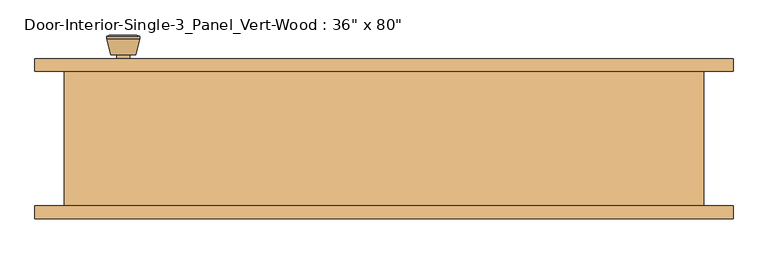
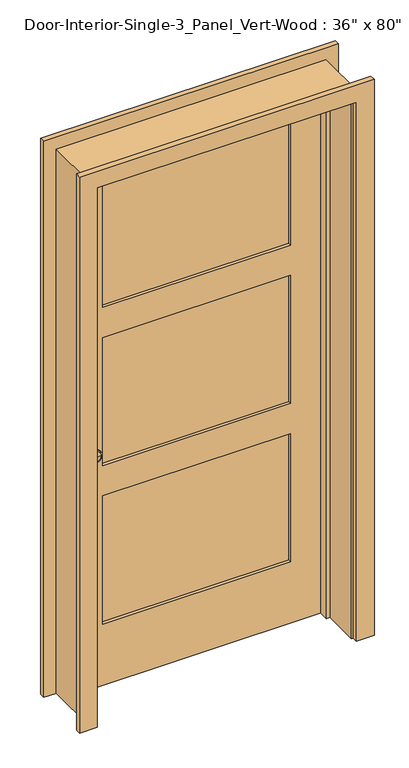
"""IFC4 building model written with IfcOpenShell, lengths in millimetres: door geometry."""

from ifc_helpers import new_model, si_unit, point, frame, frame_2d, origin, place, context, project, spatial, polyline, circle_curve, trimmed, segment, composite_curve, outline, extrude, faceted_brep, source, transform, mapped, element, save
from ifc_brep_helpers import plane_surface, cylinder_surface, revolved_surface, advanced_brep


def door_b5100634(model_context):
    return source(origin(), model_context, "Body", "SolidModel", [
        advanced_brep(
        [(-393.7, 57.5, 914.4), (-383.7, 57.5, 914.4), (-403.7, 57.5, 914.4), (-373.2241324, 8.5, 914.4), (-393.7, 8.5, 914.4), (-414.1758676, 8.5, 914.4), (-368.7, 10.3278681, 914.4), (-418.7, 10.3278681, 914.4), (-368.7, 13.7915463, 914.4), (-418.7, 13.7915463, 914.4), (-375.063764, 38.5, 914.4), (-412.336236, 38.5, 914.4), (-383.7, 38.5, 914.4), (-403.7, 38.5, 914.4)],
        [
            (0, 1),
            (1, 2, circle_curve(frame((-393.7, 57.5, 914.4), z_axis=(0.0, 1.0, 0.0), x_axis=(-1.0, 0.0, 0.0)), 10.0)),
            (2, 0),
            (2, 1, circle_curve(frame((-393.7, 57.5, 914.4), z_axis=(0.0, 1.0, 0.0), x_axis=(-1.0, 0.0, 0.0)), 10.0)),
            (3, 4),
            (4, 5),
            (5, 3, circle_curve(frame((-393.7, 8.5, 914.4), z_axis=(0.0, -1.0, 0.0), x_axis=(-1.0, 0.0, 0.0)), 20.4758676)),
            (3, 5, circle_curve(frame((-393.7, 8.5, 914.4), z_axis=(0.0, -1.0, 0.0), x_axis=(-1.0, 0.0, 0.0)), 20.4758676)),
            (6, 3),
            (5, 7),
            (7, 6, circle_curve(frame((-393.7, 10.3278681, 914.4), z_axis=(0.0, -1.0, 0.0), x_axis=(-1.0, 0.0, 0.0)), 25.0)),
            (6, 7, circle_curve(frame((-393.7, 10.3278681, 914.4), z_axis=(0.0, -1.0, 0.0), x_axis=(-1.0, 0.0, 0.0)), 25.0)),
            (8, 6),
            (7, 9),
            (9, 8, circle_curve(frame((-393.7, 13.7915463, 914.4), z_axis=(0.0, -1.0, 0.0), x_axis=(-1.0, 0.0, 0.0)), 25.0)),
            (8, 9, circle_curve(frame((-393.7, 13.7915463, 914.4), z_axis=(0.0, -1.0, 0.0), x_axis=(-1.0, 0.0, 0.0)), 25.0)),
            (10, 8),
            (9, 11),
            (11, 10, circle_curve(frame((-393.7, 38.5, 914.4), z_axis=(0.0, -1.0, 0.0), x_axis=(-1.0, 0.0, 0.0)), 18.636236)),
            (10, 11, circle_curve(frame((-393.7, 38.5, 914.4), z_axis=(0.0, -1.0, 0.0), x_axis=(-1.0, 0.0, 0.0)), 18.636236)),
            (12, 10),
            (11, 13),
            (13, 12, circle_curve(frame((-393.7, 38.5, 914.4), z_axis=(0.0, -1.0, 0.0), x_axis=(-1.0, 0.0, 0.0)), 10.0)),
            (12, 13, circle_curve(frame((-393.7, 38.5, 914.4), z_axis=(0.0, -1.0, 0.0), x_axis=(-1.0, 0.0, 0.0)), 10.0)),
            (1, 12),
            (13, 2),
        ],
        [
            plane_surface(frame((-393.7, 57.5, 914.4), z_axis=(0.0, 1.0, 0.0), x_axis=(-1.0, 0.0, 0.0))),
            plane_surface(frame((-393.7, 8.5, 914.4), z_axis=(0.0, -1.0, 0.0), x_axis=(-1.0, 0.0, 0.0))),
            revolved_surface(polyline([(-414.1758676, 8.5, 914.4), (-418.7, 10.3278681, 914.4)]), (-393.7, 57.5, 914.4), (0.0, 1.0, 0.0)),
            cylinder_surface(frame((-393.7, 57.5, 914.4), z_axis=(0.0, 1.0, 0.0), x_axis=(-1.0, 0.0, 0.0)), 25.0),
            revolved_surface(polyline([(-418.7, 13.7915463, 914.4), (-412.336236, 38.5, 914.4)]), (-393.7, 57.5, 914.4), (0.0, 1.0, 0.0)),
            plane_surface(frame((-393.7, 38.5, 914.4), z_axis=(0.0, 1.0, 0.0), x_axis=(-1.0, 0.0, 0.0))),
            cylinder_surface(frame((-393.7, 57.5, 914.4), z_axis=(0.0, 1.0, 0.0), x_axis=(-1.0, 0.0, 0.0)), 10.0),
        ],
        [
            (0, [[1, 2, 3]]),
            (0, [[-3, 4, -1]]),
            (1, [[5, 6, 7]]),
            (1, [[-6, -5, 8]]),
            (2, [[9, -7, 10, 11]]),
            (2, [[-10, -8, -9, 12]]),
            (3, [[13, -11, 14, 15]]),
            (3, [[-14, -12, -13, 16]]),
            (4, [[17, -15, 18, 19]]),
            (4, [[-18, -16, -17, 20]]),
            (5, [[21, -19, 22, 23]]),
            (5, [[-22, -20, -21, 24]]),
            (6, [[25, -23, 26, -2]]),
            (6, [[-26, -24, -25, -4]]),
        ],
    ),
        extrude(outline(composite_curve([segment(trimmed(circle_curve(frame_2d((914.4, -393.7)), 30.0), [point((914.4, -423.7))], [point((914.4, -363.7))], False, "CARTESIAN"), True, "CONTINUOUS"), segment(trimmed(circle_curve(frame_2d((914.4, -393.7)), 30.0), [point((914.4, -363.7))], [point((914.4, -423.7))], False, "CARTESIAN"), True, "CONTINUOUS")], self_intersect=False)), frame((0.0, 57.5, 0.0), z_axis=(0.0, 1.0, 0.0), x_axis=(0.0, 0.0, 1.0)), (0.0, 0.0, 1.0), 6.0),
        advanced_brep(
        [(-393.7, 104.425, 914.4), (-403.7, 104.425, 914.4), (-383.7, 104.425, 914.4), (-373.2241324, 153.425, 914.4), (-414.1758676, 153.425, 914.4), (-393.7, 153.425, 914.4), (-368.7, 151.5971319, 914.4), (-418.7, 151.5971319, 914.4), (-368.7, 148.1334537, 914.4), (-418.7, 148.1334537, 914.4), (-375.063764, 123.425, 914.4), (-412.336236, 123.425, 914.4), (-383.7, 123.425, 914.4), (-403.7, 123.425, 914.4)],
        [
            (0, 1),
            (1, 2, circle_curve(frame((-393.7, 104.425, 914.4), z_axis=(0.0, -1.0, 0.0), x_axis=(-1.0, 0.0, 0.0)), 10.0)),
            (2, 0),
            (2, 1, circle_curve(frame((-393.7, 104.425, 914.4), z_axis=(0.0, -1.0, 0.0), x_axis=(-1.0, 0.0, 0.0)), 10.0)),
            (3, 4, circle_curve(frame((-393.7, 153.425, 914.4), z_axis=(0.0, 1.0, 0.0), x_axis=(-1.0, 0.0, 0.0)), 20.4758676)),
            (4, 5),
            (5, 3),
            (4, 3, circle_curve(frame((-393.7, 153.425, 914.4), z_axis=(0.0, 1.0, 0.0), x_axis=(-1.0, 0.0, 0.0)), 20.4758676)),
            (6, 7, circle_curve(frame((-393.7, 151.5971319, 914.4), z_axis=(0.0, 1.0, 0.0), x_axis=(-1.0, 0.0, 0.0)), 25.0)),
            (7, 4),
            (3, 6),
            (7, 6, circle_curve(frame((-393.7, 151.5971319, 914.4), z_axis=(0.0, 1.0, 0.0), x_axis=(-1.0, 0.0, 0.0)), 25.0)),
            (8, 9, circle_curve(frame((-393.7, 148.1334537, 914.4), z_axis=(0.0, 1.0, 0.0), x_axis=(-1.0, 0.0, 0.0)), 25.0)),
            (9, 7),
            (6, 8),
            (9, 8, circle_curve(frame((-393.7, 148.1334537, 914.4), z_axis=(0.0, 1.0, 0.0), x_axis=(-1.0, 0.0, 0.0)), 25.0)),
            (10, 11, circle_curve(frame((-393.7, 123.425, 914.4), z_axis=(0.0, 1.0, 0.0), x_axis=(-1.0, 0.0, 0.0)), 18.636236)),
            (11, 9),
            (8, 10),
            (11, 10, circle_curve(frame((-393.7, 123.425, 914.4), z_axis=(0.0, 1.0, 0.0), x_axis=(-1.0, 0.0, 0.0)), 18.636236)),
            (12, 13, circle_curve(frame((-393.7, 123.425, 914.4), z_axis=(0.0, 1.0, 0.0), x_axis=(-1.0, 0.0, 0.0)), 10.0)),
            (13, 11),
            (10, 12),
            (13, 12, circle_curve(frame((-393.7, 123.425, 914.4), z_axis=(0.0, 1.0, 0.0), x_axis=(-1.0, 0.0, 0.0)), 10.0)),
            (1, 13),
            (12, 2),
        ],
        [
            plane_surface(frame((-393.7, 104.425, 914.4), z_axis=(0.0, -1.0, 0.0), x_axis=(-1.0, 0.0, 0.0))),
            plane_surface(frame((-393.7, 153.425, 914.4), z_axis=(0.0, 1.0, 0.0), x_axis=(-1.0, 0.0, 0.0))),
            revolved_surface(polyline([(-414.1758676, 153.425, 914.4), (-418.7, 151.5971319, 914.4)]), (-393.7, 104.425, 914.4), (0.0, -1.0, 0.0)),
            cylinder_surface(frame((-393.7, 104.425, 914.4), z_axis=(0.0, -1.0, 0.0), x_axis=(-1.0, 0.0, 0.0)), 25.0),
            revolved_surface(polyline([(-418.7, 148.1334537, 914.4), (-412.336236, 123.425, 914.4)]), (-393.7, 104.425, 914.4), (0.0, -1.0, 0.0)),
            plane_surface(frame((-393.7, 123.425, 914.4), z_axis=(0.0, -1.0, 0.0), x_axis=(-1.0, 0.0, 0.0))),
            cylinder_surface(frame((-393.7, 104.425, 914.4), z_axis=(0.0, -1.0, 0.0), x_axis=(-1.0, 0.0, 0.0)), 10.0),
        ],
        [
            (0, [[1, 2, 3]]),
            (0, [[-3, 4, -1]]),
            (1, [[5, 6, 7]]),
            (1, [[8, -7, -6]]),
            (2, [[9, 10, -5, 11]]),
            (2, [[12, -11, -8, -10]]),
            (3, [[13, 14, -9, 15]]),
            (3, [[16, -15, -12, -14]]),
            (4, [[17, 18, -13, 19]]),
            (4, [[20, -19, -16, -18]]),
            (5, [[21, 22, -17, 23]]),
            (5, [[24, -23, -20, -22]]),
            (6, [[-2, 25, -21, 26]]),
            (6, [[-4, -26, -24, -25]]),
        ],
    ),
        extrude(outline(composite_curve([segment(trimmed(circle_curve(frame_2d((914.4, -393.7)), 30.0), [point((914.4, -423.7))], [point((914.4, -363.7))], False, "CARTESIAN"), True, "CONTINUOUS"), segment(trimmed(circle_curve(frame_2d((914.4, -393.7)), 30.0), [point((914.4, -363.7))], [point((914.4, -423.7))], False, "CARTESIAN"), True, "CONTINUOUS")], self_intersect=False)), frame((0.0, 98.425, 0.0), z_axis=(0.0, 1.0, 0.0), x_axis=(0.0, 0.0, 1.0)), (0.0, 0.0, 1.0), 6.0),
        extrude(outline(polyline([(336.55, 75.1416667), (-336.55, 75.1416667), (-336.55, 86.7833333), (336.55, 86.7833333), (336.55, 75.1416667)])), frame((0.0, 0.0, 1428.75), z_axis=(0.0, 0.0, 1.0), x_axis=(1.0, 0.0, 0.0)), (0.0, 0.0, 1.0), 484.1875),
        extrude(outline(polyline([(336.55, 75.1416667), (-336.55, 75.1416667), (-336.55, 86.7833333), (336.55, 86.7833333), (336.55, 75.1416667)])), frame((0.0, 0.0, 231.775), z_axis=(0.0, 0.0, 1.0), x_axis=(1.0, 0.0, 0.0)), (0.0, 0.0, 1.0), 484.1875),
        extrude(outline(polyline([(336.55, 75.1416667), (-336.55, 75.1416667), (-336.55, 86.7833333), (336.55, 86.7833333), (336.55, 75.1416667)])), frame((0.0, 0.0, 830.2625), z_axis=(0.0, 0.0, 1.0), x_axis=(1.0, 0.0, 0.0)), (0.0, 0.0, 1.0), 484.1875),
        extrude(outline(polyline([(2032.0, -457.2), (0.0, -457.2), (0.0, 457.2), (2032.0, 457.2), (2032.0, -457.2)]), holes=[polyline([(1912.9375, -336.55), (1912.9375, 336.55), (1428.75, 336.55), (1428.75, -336.55), (1912.9375, -336.55)]), polyline([(715.9625, -336.55), (715.9625, 336.55), (231.775, 336.55), (231.775, -336.55), (715.9625, -336.55)]), polyline([(1314.45, -336.55), (1314.45, 336.55), (830.2625, 336.55), (830.2625, -336.55), (1314.45, -336.55)])]), frame((0.0, 63.5, 0.0), z_axis=(0.0, 1.0, 0.0), x_axis=(0.0, 0.0, 1.0)), (0.0, 0.0, 1.0), 34.925),
        faceted_brep([(482.6, 98.425, 0.0), (482.6, -104.775, 0.0), (457.2, -104.775, 0.0), (457.2, 28.575, 0.0), (444.5, 28.575, 0.0), (444.5, 63.5, 0.0), (457.2, 63.5, 0.0), (457.2, 98.425, 0.0), (482.6, 98.425, 2057.4), (482.6, -104.775, 2057.4), (-482.6, -104.775, 2057.4), (-482.6, -104.775, 0.0), (-457.2, -104.775, 0.0), (-457.2, -104.775, 2032.0), (457.2, -104.775, 2032.0), (457.2, 28.575, 2032.0), (-457.2, 28.575, 2032.0), (-457.2, 28.575, 0.0), (-444.5, 28.575, 0.0), (-444.5, 28.575, 2019.3), (444.5, 28.575, 2019.3), (444.5, 63.5, 2019.3), (-444.5, 63.5, 2019.3), (-444.5, 63.5, 0.0), (-457.2, 63.5, 0.0), (-457.2, 63.5, 2032.0), (457.2, 63.5, 2032.0), (457.2, 98.425, 2032.0), (-457.2, 98.425, 2032.0), (-457.2, 98.425, 0.0), (-482.6, 98.425, 0.0), (-482.6, 98.425, 2057.4)], [[[0, 1, 2, 3, 4, 5, 6, 7]], [[1, 0, 8, 9]], [[2, 1, 9, 10, 11, 12, 13, 14]], [[3, 2, 14, 15]], [[4, 3, 15, 16, 17, 18, 19, 20]], [[5, 4, 20, 21]], [[6, 5, 21, 22, 23, 24, 25, 26]], [[7, 6, 26, 27]], [[0, 7, 27, 28, 29, 30, 31, 8]], [[9, 8, 31, 10]], [[15, 14, 13, 16]], [[21, 20, 19, 22]], [[27, 26, 25, 28]], [[30, 29, 24, 23, 18, 17, 12, 11]], [[10, 31, 30, 11]], [[16, 13, 12, 17]], [[22, 19, 18, 23]], [[28, 25, 24, 29]]]),
        extrude(outline(polyline([(0.0, 463.55), (0.0, 527.05), (2101.85, 527.05), (2101.85, -527.05), (0.0, -527.05), (0.0, -463.55), (2038.35, -463.55), (2038.35, 463.55), (0.0, 463.55)])), frame((0.0, -123.825, 0.0), z_axis=(0.0, 1.0, 0.0), x_axis=(0.0, 0.0, 1.0)), (0.0, 0.0, 1.0), 19.05),
        extrude(outline(polyline([(0.0, 463.55), (0.0, 527.05), (2101.85, 527.05), (2101.85, -527.05), (0.0, -527.05), (0.0, -463.55), (2038.35, -463.55), (2038.35, 463.55), (0.0, 463.55)])), frame((0.0, 98.425, 0.0), z_axis=(0.0, 1.0, 0.0), x_axis=(0.0, 0.0, 1.0)), (0.0, 0.0, 1.0), 19.05),
    ])


if __name__ == "__main__":
    model = new_model("IFC4")
    model_context = context("Model", 3, world=origin())
    ifc_project = project(units=[si_unit("LENGTHUNIT", "METRE", prefix="MILLI")], contexts=[model_context])
    site = spatial("IfcSite", under=ifc_project)
    building = spatial("IfcBuilding", under=site)
    placement = place(None, origin())
    door_shape = door_b5100634(model_context)
    element("IfcDoor", 1, ObjectType="Door-Interior-Single-3_Panel_Vert-Wood : 36\" x 80\"", at=placement, inside=building, context=model_context, shape_type="MappedRepresentation", body=[
        mapped(door_shape, transform((0.0, 0.0, 0.0), x_axis=(1.0, 0.0, 0.0), y_axis=(0.0, 1.0, 0.0), z_axis=(0.0, 0.0, 1.0))),
    ])
    save(model, "model.ifc")

# Revit data of these elements
# Type "Door-Interior-Single-3_Panel_Vert-Wood : 36\" x 80\""
#   Type Mark = "9"
#   Assembly Code = "C1020300"
#   Analytic Construction = "Wooden"
#   Top Rail = 0' - 4 11/16"
#   Thickness = 0' - 1 3/8"
#   Thermal Resistance (R) = 0.455703 (m²·K)/W
#   Swing Angle [instance default] = 90.00°
#   Stiles = 0' - 4 3/4"
#   Rough Width = 3' - 2"
#   Rough Height = 6' - 9"
#   Intermediate Rail = 0' - 4 1/2"
#   Height = 6' - 8"
#   Width = 3' - 0"
#   Heat Transfer Coefficient (U) = 2.19465 W/(m²·K)
#   Bottom Rail = 0' - 9 1/8"
#   Trim Material = Cherry
#   Panel Material = Cherry
#   Frame Material = Cherry
#   Door Handle Material = Aluminum
#   Visual Light Transmittance = 0
#   Solar Heat Gain Coefficient = 0
#   Wall Closure = (empty or 0)
#   Function = (empty or 0)
# Element 1 (IfcDoor, "Door-Interior-Single-3_Panel_Vert-Wood : 36\" x 80\"")
#   Materials on its faces: "Cherry", "Aluminum"
# Materials
#   "Cherry": class "Wood", colour RGB 226 177 128, transparency 0, Description = "Prunus Serotina", Cost = 0
#   "Aluminum": class "Metal", colour RGB 247 247 247, transparency 0, Description = "Aluminum 6061", Cost = 0
